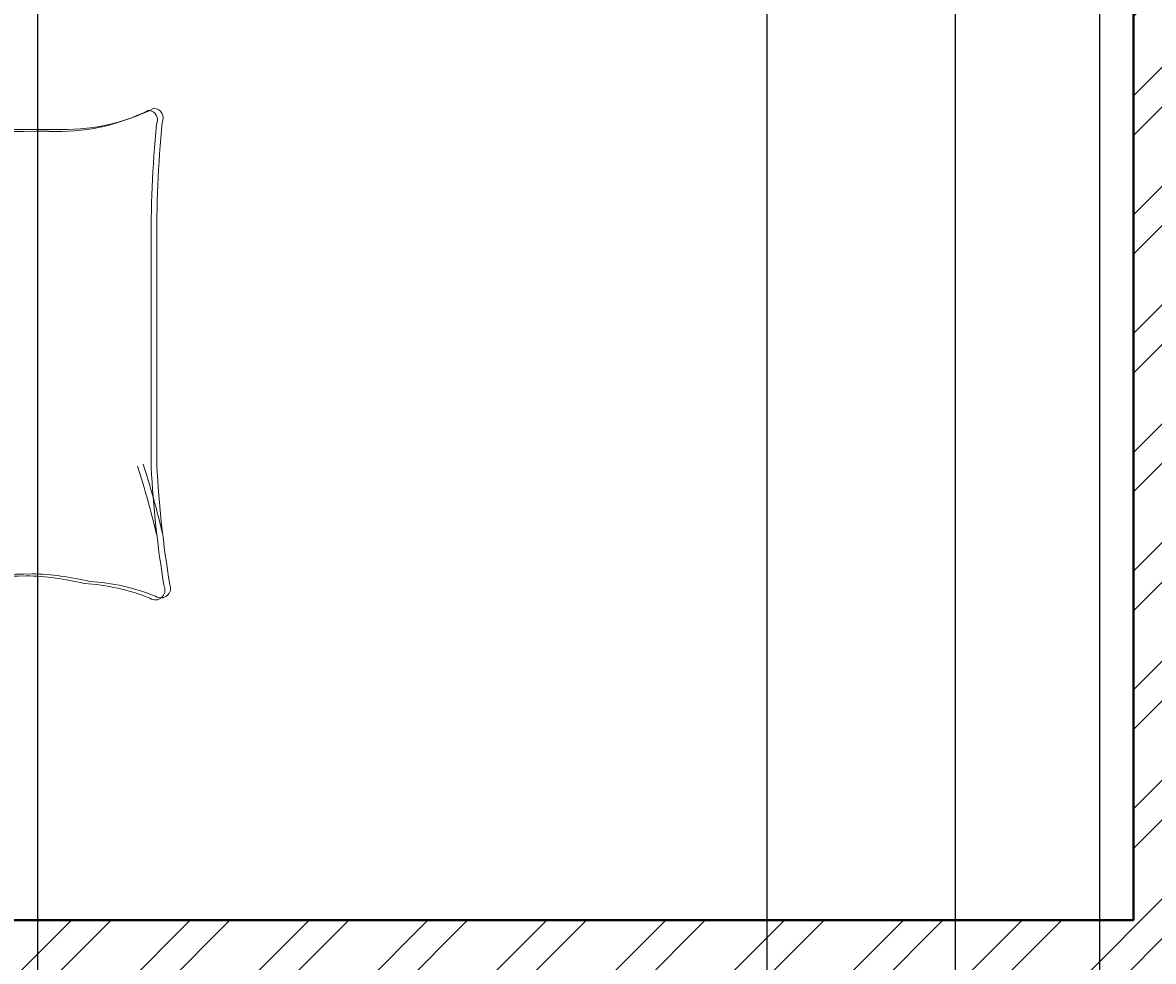
# Model space of a CAD drawing. Units: inches. Extents: x 1601 to 2297, y 1496 to 2631.
# Tile 36 of 57: x 1763 to 1891, y 2141 to 2247. Entities that reach past the tile are written whole.
import ezdxf

# ---------------------------------------------------------------- set-up
doc = ezdxf.new("R2010")
doc.units = ezdxf.units.IN
for name, color, linetype, lineweight in [('A-ANNO-DIMS', 2, 'Continuous', 18), ('A-FURN', 8, 'Continuous', 18), ('A-WALL', 7, 'Continuous', 40), ('A-WALL-PATT', 215, 'Continuous', 13)]:
    doc.layers.add(name, color=color, linetype=linetype, lineweight=lineweight)
doc.styles.get("Standard").update_dxf_attribs({"font": 'arial.ttf'})
doc.dimstyles.get("Standard").update_dxf_attribs({"dimtxt": 0.18, "dimasz": 0.18, "dimexe": 0.18, "dimexo": 0.0625, "dimgap": 0.09, "dimtad": 0, "dimtih": 1, "dimtoh": 1, "dimdec": 4, "dimzin": 0, "dimdsep": 46, "dimtxsty": 'Standard', "dimcen": 0.09, "dimadec": 0, "dimazin": 0, "dimtfac": 1, "dimtdec": 4, "dimtofl": 0, "dimtmove": 0, "dimatfit": 3, "dimfxl": 1, "dimtolj": 1, "dimtzin": 0, "dimarcsym": 0})

# ---------------------------------------------------------------- blocks, each defined once
blk = doc.blocks.new('BED-DOUBLE')
for p, q in [((27.75, 52.87), (24.5, 49.16)), ((27.75, 52.87), (24.5, 49.16)), ((27.75, 52.87), (24.5, 49.16)), ((27.75, 52.87), (24.5, 49.16)), ((28.39, 53.1), (25.13, 49.39)), ((28.39, 53.1), (25.13, 49.39)), ((28.39, 53.1), (25.13, 49.39)), ((28.39, 53.1), (25.13, 49.39)), ((29.49, 52.95), (27.75, 52.87, 3.87)), ((29.49, 52.95), (27.75, 52.87, 3.87)), ((29.49, 52.95), (27.75, 52.87, 3.87)), ((29.49, 52.95), (27.75, 52.87, 3.87)), ((28.36, 51.33), (27.75, 52.87)), ((28.36, 51.33), (27.75, 52.87)), ((28.36, 51.33), (27.75, 52.87)), ((28.36, 51.33), (27.75, 52.87)), ((30.13, 53.18), (28.39, 53.1, 3.87)), ((30.13, 53.18), (28.39, 53.1, 3.87)), ((30.13, 53.17), (28.39, 53.1, 3.87)), ((30.13, 53.17), (28.39, 53.1, 3.87)), ((29, 51.56), (28.39, 53.1)), ((29, 51.56), (28.39, 53.1)), ((29, 51.56), (28.39, 53.1)), ((29, 51.56), (28.39, 53.1)), ((0, 51.49), (0.64, 51.49)), ((0, 3.47), (0, 51.49)), ((0, 51.49), (0.64, 51.49)), ((0, 3.47), (0, 51.49)), ((0.64, 51.49), (27.25, 51.49)), ((0.64, 51.49), (27.25, 51.49)), ((0.64, 51.49), (27.25, 51.49)), ((0.64, 51.49), (27.25, 51.49)), ((2.17, 3.7), (2.17, 51.49)), ((2.17, 3.7), (2.17, 51.49)), ((2.17, 3.7), (2.17, 51.49)), ((2.17, 3.7), (2.17, 51.49)), ((28.06, 48.23), (28.36, 51.33)), ((28.06, 48.23), (28.36, 51.33)), ((28.06, 48.23), (28.36, 51.33)), ((28.06, 48.23), (28.36, 51.33)), ((28.69, 48.46), (29, 51.56)), ((28.69, 48.46), (29, 51.56)), ((28.69, 48.46), (29, 51.56)), ((28.69, 48.46), (29, 51.56)), ((0, 51.27), (26.61, 51.27)), ((0, 51.27), (26.61, 51.27)), ((0, 51.26), (26.61, 51.26)), ((0, 51.26), (26.61, 51.26)), ((1.53, 3.47), (1.53, 51.27)), ((1.53, 3.47), (1.53, 51.27)), ((1.53, 3.47), (1.53, 51.26)), ((1.53, 3.47), (1.53, 51.26)), ((2.56, 50.11), (2.46, 44.71)), ((2.56, 50.11), (2.46, 44.71)), ((2.56, 50.11), (2.46, 44.71)), ((2.56, 50.11), (2.46, 44.71)), ((2.56, 50.11), (5.77, 49.73)), ((2.56, 50.11), (5.77, 49.73)), ((2.56, 50.11), (5.77, 49.73)), ((2.56, 50.11), (5.77, 49.73)), ((3.2, 50.34), (3.1, 44.94)), ((3.2, 50.34), (3.1, 44.94)), ((3.2, 50.34), (3.1, 44.94)), ((3.2, 50.34), (3.1, 44.94)), ((3.2, 50.34), (6.41, 49.96)), ((3.2, 50.34), (6.41, 49.96)), ((3.2, 50.34), (6.41, 49.96)), ((3.2, 50.34), (6.41, 49.96)), ((5.77, 49.73), (8.34, 50.33)), ((5.77, 49.73), (8.34, 50.33)), ((5.77, 49.73), (8.34, 50.33)), ((5.77, 49.73), (8.34, 50.33)), ((6.41, 49.96), (8.98, 50.56)), ((6.41, 49.96), (8.98, 50.56)), ((6.41, 49.96), (8.98, 50.56)), ((6.41, 49.96), (8.98, 50.56)), ((11.83, 50.11), (8.26, 49.31)), ((11.83, 50.11), (8.26, 49.31)), ((11.83, 50.11), (8.26, 49.31)), ((11.83, 50.11), (8.26, 49.31)), ((8.34, 50.33), (9.38, 49.81)), ((8.34, 50.33), (9.38, 49.81)), ((8.34, 50.33), (9.38, 49.81)), ((8.34, 50.33), (9.38, 49.81)), ((12.47, 50.34), (8.9, 49.54)), ((12.47, 50.34), (8.9, 49.54)), ((12.47, 50.34), (8.9, 49.54)), ((12.47, 50.34), (8.9, 49.54)), ((8.98, 50.56), (10.02, 50.04)), ((8.98, 50.56), (10.02, 50.04)), ((8.98, 50.56), (10.02, 50.04)), ((8.98, 50.56), (10.02, 50.04)), ((13.43, 49.92), (11.83, 50.11)), ((13.43, 49.92), (11.83, 50.11)), ((13.43, 49.92), (11.83, 50.11)), ((13.43, 49.92), (11.83, 50.11)), ((14.07, 50.15), (12.47, 50.34)), ((14.07, 50.15), (12.47, 50.34)), ((14.07, 50.15), (12.47, 50.34)), ((14.07, 50.15), (12.47, 50.34)), ((16.57, 50.7), (13.43, 49.92)), ((16.57, 50.7), (13.43, 49.92)), ((16.57, 50.7), (13.43, 49.92)), ((16.57, 50.7), (13.43, 49.92)), ((17.21, 50.93), (14.07, 50.15)), ((17.21, 50.93), (14.07, 50.15)), ((17.21, 50.93), (14.07, 50.15)), ((17.21, 50.93), (14.07, 50.15)), ((16.17, 45.57), (16.57, 50.7)), ((16.17, 45.57), (16.57, 50.7)), ((16.17, 45.57), (16.57, 50.7)), ((16.17, 45.57), (16.57, 50.7)), ((16.81, 45.79), (17.21, 50.93)), ((16.81, 45.79), (17.21, 50.93)), ((16.81, 45.79), (17.21, 50.93)), ((16.81, 45.79), (17.21, 50.93)), ((8.26, 49.31), (5.58, 48.13)), ((8.26, 49.31), (5.58, 48.13)), ((8.26, 49.31), (5.58, 48.13)), ((8.26, 49.31), (5.58, 48.13)), ((8.9, 49.54), (6.22, 48.36)), ((8.9, 49.54), (6.22, 48.36)), ((8.9, 49.54), (6.22, 48.36)), ((8.9, 49.54), (6.22, 48.36)), ((24.5, 49.16), (22.33, 46.22)), ((24.5, 49.16), (22.33, 46.22)), ((24.5, 49.16), (22.33, 46.22)), ((24.5, 49.16), (22.33, 46.22)), ((25.13, 49.39), (22.97, 46.45)), ((25.13, 49.39), (22.97, 46.45)), ((25.13, 49.39), (22.97, 46.45)), ((25.13, 49.39), (22.97, 46.45)), ((28.36, 44.36), (28.06, 48.23)), ((28.36, 44.36), (28.06, 48.23)), ((28.36, 44.36), (28.06, 48.23)), ((28.36, 44.36), (28.06, 48.23)), ((29, 44.59), (28.69, 48.46)), ((29, 44.59), (28.69, 48.46)), ((29, 44.59), (28.69, 48.46)), ((29, 44.59), (28.69, 48.46)), ((22.33, 46.22), (20.32, 40.64)), ((22.33, 46.22), (20.32, 40.64)), ((22.33, 46.22), (20.32, 40.64)), ((22.33, 46.22), (20.32, 40.64)), ((22.97, 46.45), (20.96, 40.87)), ((22.97, 46.45), (20.96, 40.87)), ((22.97, 46.45), (20.96, 40.87)), ((22.97, 46.45), (20.96, 40.87)), ((2.46, 44.71), (2.54, 45.71)), ((2.46, 44.71), (2.54, 45.71)), ((2.46, 44.71), (2.54, 45.71)), ((2.46, 44.71), (2.54, 45.71)), ((2.54, 45.71), (3.07, 41.91)), ((2.54, 45.71), (3.07, 41.91)), ((2.54, 45.71), (3.07, 41.91)), ((2.54, 45.71), (3.07, 41.91)), ((3.1, 44.94), (3.18, 45.94)), ((3.1, 44.94), (3.18, 45.94)), ((3.1, 44.94), (3.18, 45.94)), ((3.1, 44.94), (3.18, 45.94)), ((3.18, 45.94), (3.71, 42.14)), ((3.18, 45.94), (3.71, 42.14)), ((3.18, 45.94), (3.71, 42.14)), ((3.18, 45.94), (3.71, 42.14)), ((16.73, 43.61), (16.17, 45.57)), ((16.73, 43.61), (16.17, 45.57)), ((16.73, 43.61), (16.17, 45.57)), ((16.73, 43.61), (16.17, 45.57)), ((17.37, 43.83), (16.81, 45.79)), ((17.37, 43.83), (16.81, 45.79)), ((17.37, 43.83), (16.81, 45.79)), ((17.37, 43.83), (16.81, 45.79)), ((16.3, 36.6), (16.73, 43.61)), ((16.3, 36.6), (16.73, 43.61)), ((16.3, 36.6), (16.73, 43.61)), ((16.3, 36.6), (16.73, 43.61)), ((16.93, 36.82), (17.37, 43.83)), ((16.93, 36.82), (17.37, 43.83)), ((16.93, 36.82), (17.37, 43.83)), ((16.93, 36.82), (17.37, 43.83)), ((28.83, 40.95), (28.36, 44.36)), ((28.83, 40.95), (28.36, 44.36)), ((28.83, 40.95), (28.36, 44.36)), ((28.83, 40.95), (28.36, 44.36)), ((29.47, 41.18), (29, 44.59)), ((29.47, 41.18), (29, 44.59)), ((29.47, 41.18), (29, 44.59)), ((29.47, 41.18), (29, 44.59)), ((3.07, 41.91), (4.42, 36.49)), ((3.07, 41.91), (4.42, 36.49)), ((3.07, 41.91), (4.42, 36.49)), ((3.07, 41.91), (4.42, 36.49)), ((3.71, 42.14), (5.06, 36.72)), ((3.71, 42.14), (5.06, 36.72)), ((3.71, 42.14), (5.06, 36.72)), ((3.71, 42.14), (5.06, 36.72)), ((30.4, 39.17), (29.47, 41.18)), ((30.4, 39.17), (29.47, 41.18)), ((30.4, 39.17), (29.47, 41.18)), ((30.4, 39.17), (29.47, 41.18)), ((20.32, 40.64), (17.38, 32.31)), ((20.32, 40.64), (17.38, 32.31)), ((20.32, 40.64), (17.38, 32.31)), ((20.32, 40.64), (17.38, 32.31)), ((20.96, 40.87), (18.02, 32.53)), ((20.96, 40.87), (18.02, 32.53)), ((20.96, 40.87), (18.02, 32.53)), ((20.96, 40.87), (18.02, 32.53)), ((29.76, 38.94), (28.83, 40.95)), ((29.76, 38.94), (28.83, 40.95)), ((29.76, 38.94), (28.83, 40.95)), ((29.76, 38.94), (28.83, 40.95)), ((79.88, 15.29), (79.88, 39.91)), ((79.88, 15.29), (79.88, 39.91)), ((79.88, 15.29), (79.88, 39.91)), ((79.88, 15.29), (79.88, 39.91)), ((3.67, 39.2), (3.08, 37.14)), ((3.67, 39.2), (3.08, 37.13)), ((3.67, 39.2), (3.08, 37.14)), ((3.67, 39.2), (3.08, 37.13)), ((4.31, 39.43), (3.72, 37.36)), ((4.31, 39.43), (3.72, 37.36)), ((4.31, 39.43), (3.72, 37.36)), ((4.31, 39.43), (3.72, 37.36)), ((30.38, 36.46), (29.76, 38.94)), ((30.38, 36.46), (29.76, 38.94)), ((30.38, 36.46), (29.76, 38.94)), ((30.38, 36.46), (29.76, 38.94)), ((31.02, 36.69), (30.4, 39.17)), ((31.02, 36.69), (30.4, 39.17)), ((31.02, 36.69), (30.4, 39.17)), ((31.02, 36.69), (30.4, 39.17)), ((79.24, 15.06), (79.24, 39.68)), ((79.24, 15.06), (79.24, 39.68)), ((79.24, 15.06), (79.24, 39.68)), ((79.24, 15.06), (79.24, 39.68)), ((3.72, 37.36), (3.18, 34.43)), ((3.72, 37.36), (3.18, 34.43)), ((3.72, 37.36), (3.18, 34.43)), ((3.72, 37.36), (3.18, 34.43)), ((3.08, 37.14), (2.54, 34.2)), ((3.08, 37.14), (2.54, 34.2)), ((3.08, 37.13), (2.54, 34.2)), ((3.08, 37.13), (2.54, 34.2)), ((15.63, 32.56), (16.3, 36.6)), ((15.63, 32.56), (16.3, 36.6)), ((15.63, 32.56), (16.3, 36.6)), ((15.63, 32.56), (16.3, 36.6)), ((16.27, 32.79), (16.93, 36.82)), ((16.27, 32.79), (16.93, 36.82)), ((16.27, 32.79), (16.93, 36.82)), ((16.27, 32.79), (16.93, 36.82)), ((23.88, 34.45), (28.36, 36.15)), ((23.88, 34.45), (28.36, 36.15)), ((23.88, 34.45), (28.36, 36.15)), ((23.88, 34.45), (28.36, 36.15)), ((24.52, 34.68), (29, 36.38)), ((24.52, 34.68), (29, 36.38)), ((24.52, 34.68), (29, 36.38)), ((24.52, 34.68), (29, 36.38)), ((28.36, 36.15), (30.38, 36.46)), ((28.36, 36.15), (30.38, 36.46)), ((28.36, 36.15), (30.38, 36.46)), ((28.36, 36.15), (30.38, 36.46)), ((29, 36.38), (31.02, 36.69)), ((29, 36.38), (31.02, 36.69)), ((29, 36.38), (31.02, 36.69)), ((29, 36.38), (31.02, 36.69)), ((18.02, 30.49), (24.52, 34.68)), ((18.02, 30.49), (24.52, 34.68)), ((18.02, 30.49), (24.52, 34.68)), ((18.02, 30.49), (24.52, 34.68)), ((2.54, 34.2), (2.56, 33.88)), ((2.54, 34.2), (2.56, 33.88)), ((2.54, 34.2), (2.56, 33.88)), ((2.54, 34.2), (2.56, 33.88)), ((2.56, 33.88), (2.98, 29.46)), ((2.56, 33.88), (2.98, 29.46)), ((2.56, 33.88), (2.98, 29.46)), ((2.56, 33.88), (2.98, 29.46)), ((3.18, 34.43), (3.2, 34.11)), ((3.18, 34.43), (3.2, 34.11)), ((3.18, 34.43), (3.2, 34.11)), ((3.18, 34.43), (3.2, 34.11)), ((3.2, 34.11), (3.62, 29.68)), ((3.2, 34.11), (3.62, 29.68)), ((3.2, 34.11), (3.62, 29.68)), ((3.2, 34.11), (3.62, 29.68)), ((16.74, 30.75), (15.45, 33.82)), ((16.74, 30.75), (15.45, 33.82)), ((16.74, 30.75), (15.45, 33.82)), ((16.74, 30.75), (15.45, 33.82)), ((17.38, 30.98), (16.09, 34.05)), ((17.38, 30.98), (16.09, 34.05)), ((17.38, 30.98), (16.09, 34.05)), ((17.38, 30.98), (16.09, 34.05)), ((17.38, 30.26), (23.88, 34.45)), ((17.38, 30.26), (23.88, 34.45)), ((17.38, 30.26), (23.88, 34.45)), ((17.38, 30.26), (23.88, 34.45)), ((17.53, 28.53), (17.38, 30.98)), ((17.53, 28.53), (17.38, 30.98)), ((17.53, 28.53), (17.38, 30.98)), ((17.53, 28.53), (17.38, 30.98)), ((3.62, 29.68), (3.13, 28.21)), ((3.62, 29.68), (3.13, 28.2)), ((3.62, 29.68), (3.13, 28.21)), ((3.62, 29.68), (3.13, 28.2)), ((16.89, 28.3), (16.74, 30.75)), ((16.89, 28.3), (16.74, 30.75)), ((16.89, 28.3), (16.74, 30.75)), ((16.89, 28.3), (16.74, 30.75)), ((2.98, 29.46), (2.49, 27.98)), ((2.98, 29.46), (2.49, 27.98)), ((2.98, 29.46), (2.49, 27.98)), ((2.98, 29.46), (2.49, 27.98)), ((3.13, 28.21), (8.51, 27.96)), ((3.13, 28.21), (8.51, 27.96)), ((3.13, 28.2), (8.51, 27.96)), ((3.13, 28.2), (8.51, 27.96)), ((13.02, 27.66), (14.86, 28.36)), ((13.02, 27.66), (14.86, 28.36)), ((13.02, 27.66), (14.86, 28.36)), ((13.02, 27.66), (14.86, 28.36)), ((14.22, 28.13), (16.89, 28.3)), ((14.22, 28.13), (16.89, 28.3)), ((14.22, 28.13), (16.89, 28.3)), ((14.22, 28.13), (16.89, 28.3)), ((14.86, 28.36), (17.53, 28.53)), ((14.86, 28.36), (17.53, 28.53)), ((14.86, 28.36), (17.53, 28.53)), ((14.86, 28.36), (17.53, 28.53)), ((2.49, 27.98), (7.87, 27.73)), ((2.49, 27.98), (7.87, 27.73)), ((2.49, 27.98), (7.87, 27.73)), ((2.49, 27.98), (7.87, 27.73)), ((7.22, 26.56), (10.4, 27.14)), ((7.22, 26.56), (10.4, 27.14)), ((7.22, 26.56), (10.4, 27.14)), ((7.22, 26.56), (10.4, 27.14)), ((7.86, 26.79), (11.04, 27.37)), ((7.86, 26.79), (11.04, 27.37)), ((7.86, 26.79), (11.04, 27.37)), ((7.86, 26.79), (11.04, 27.37)), ((7.87, 27.73), (11.08, 27.35)), ((7.87, 27.73), (11.08, 27.35)), ((7.87, 27.73), (11.08, 27.35)), ((7.87, 27.73), (11.08, 27.35)), ((8.51, 27.96), (11.72, 27.58)), ((8.51, 27.96), (11.72, 27.58)), ((8.51, 27.96), (11.72, 27.58)), ((8.51, 27.96), (11.72, 27.58)), ((10.4, 27.14), (11.7, 27.14)), ((10.4, 27.14), (11.7, 27.14)), ((10.4, 27.14), (11.7, 27.14)), ((10.4, 27.14), (11.7, 27.14)), ((11.04, 27.37), (12.34, 27.37)), ((11.04, 27.37), (12.34, 27.37)), ((11.04, 27.37), (12.34, 27.37)), ((11.04, 27.37), (12.34, 27.37)), ((11.08, 27.35), (12.38, 27.44)), ((11.08, 27.35), (12.38, 27.44)), ((11.08, 27.35), (12.38, 27.44)), ((11.08, 27.35), (12.38, 27.44)), ((11.7, 27.14), (13.58, 26.56)), ((11.7, 27.14), (13.58, 26.56)), ((11.7, 27.14), (13.58, 26.56)), ((11.7, 27.14), (13.58, 26.56)), ((11.72, 27.58), (13.02, 27.66)), ((11.72, 27.58), (13.02, 27.66)), ((11.72, 27.58), (13.02, 27.66)), ((11.72, 27.58), (13.02, 27.66)), ((12.34, 27.37), (14.22, 26.79)), ((12.34, 27.37), (14.22, 26.79)), ((12.34, 27.37), (14.22, 26.79)), ((12.34, 27.37), (14.22, 26.79)), ((12.38, 27.44), (14.22, 28.13)), ((12.38, 27.44), (14.22, 28.13)), ((12.38, 27.44), (14.22, 28.13)), ((12.38, 27.44), (14.22, 28.13)), ((1.87, 25.98), (7.22, 26.56)), ((1.87, 25.98), (7.22, 26.56)), ((1.87, 25.98), (7.22, 26.56)), ((1.87, 25.98), (7.22, 26.56)), ((2.45, 24.54), (1.87, 25.98)), ((2.45, 24.54), (1.87, 25.98)), ((2.45, 24.54), (1.87, 25.98)), ((2.45, 24.54), (1.87, 25.98)), ((2.51, 26.21), (7.86, 26.79)), ((2.51, 26.21), (7.86, 26.79)), ((2.51, 26.21), (7.86, 26.79)), ((2.51, 26.21), (7.86, 26.79)), ((3.09, 24.77), (2.51, 26.21)), ((3.09, 24.76), (2.51, 26.21)), ((3.09, 24.77), (2.51, 26.21)), ((3.09, 24.76), (2.51, 26.21)), ((13.58, 26.56), (16.26, 26.56)), ((13.58, 26.56), (16.26, 26.56)), ((13.58, 26.56), (16.26, 26.56)), ((13.58, 26.56), (16.26, 26.56)), ((14.22, 26.79), (16.9, 26.79)), ((14.22, 26.79), (16.9, 26.79)), ((14.22, 26.79), (16.9, 26.79)), ((14.22, 26.79), (16.9, 26.79)), ((16.26, 26.56), (16.26, 24.1)), ((16.26, 26.56), (16.26, 24.1)), ((16.26, 26.56), (16.26, 24.1)), ((16.26, 26.56), (16.26, 24.1)), ((16.9, 26.79), (16.9, 24.33)), ((16.9, 26.79), (16.9, 24.33)), ((16.9, 26.79), (16.9, 24.33)), ((16.9, 26.79), (16.9, 24.33)), ((2.3, 20.09), (2.45, 24.54)), ((2.3, 20.09), (2.45, 24.54)), ((2.3, 20.09), (2.45, 24.54)), ((2.3, 20.09), (2.45, 24.54)), ((2.94, 20.32), (3.09, 24.77)), ((2.94, 20.32), (3.09, 24.77)), ((2.94, 20.32), (3.09, 24.76)), ((2.94, 20.32), (3.09, 24.76)), ((16.17, 19.38), (16.57, 24.52)), ((16.17, 19.38), (16.57, 24.52)), ((16.17, 19.38), (16.57, 24.52)), ((16.17, 19.38), (16.57, 24.52)), ((16.81, 19.61), (17.21, 24.74)), ((16.81, 19.61), (17.21, 24.74)), ((16.81, 19.61), (17.21, 24.74)), ((16.81, 19.61), (17.21, 24.74)), ((16.26, 24.1), (15.17, 20.96)), ((16.26, 24.1), (15.17, 20.96)), ((16.26, 24.1), (15.17, 20.96)), ((16.26, 24.1), (15.17, 20.96)), ((16.9, 24.33), (15.81, 21.19)), ((16.9, 24.33), (15.81, 21.19)), ((16.9, 24.33), (15.81, 21.19)), ((16.9, 24.33), (15.81, 21.19)), ((2.3, 19.77), (2.3, 20.09)), ((2.3, 19.77), (2.3, 20.09)), ((2.3, 19.77), (2.3, 20.09)), ((2.3, 19.77), (2.3, 20.09)), ((3.03, 16.88), (2.3, 19.77)), ((3.03, 16.88), (2.3, 19.77)), ((3.03, 16.88), (2.3, 19.77)), ((3.03, 16.88), (2.3, 19.77)), ((2.94, 20), (2.94, 20.32)), ((2.94, 20), (2.94, 20.32)), ((2.94, 20), (2.94, 20.32)), ((2.94, 20), (2.94, 20.32)), ((3.67, 17.11), (2.94, 20)), ((3.67, 17.11), (2.94, 20)), ((3.67, 17.11), (2.94, 20)), ((3.67, 17.11), (2.94, 20)), ((16.73, 17.42), (16.17, 19.38)), ((16.73, 17.42), (16.17, 19.38)), ((16.73, 17.42), (16.17, 19.38)), ((16.73, 17.42), (16.17, 19.38)), ((17.37, 17.65), (16.81, 19.61)), ((17.37, 17.65), (16.81, 19.61)), ((17.37, 17.65), (16.81, 19.61)), ((17.37, 17.65), (16.81, 19.61)), ((3.75, 14.85), (3.03, 16.88)), ((3.75, 14.85), (3.03, 16.88)), ((3.75, 14.85), (3.03, 16.88)), ((3.75, 14.85), (3.03, 16.88)), ((3.32, 12.11), (4.33, 17.6)), ((3.32, 12.11), (4.33, 17.6)), ((3.32, 12.11), (4.33, 17.6)), ((3.32, 12.11), (4.33, 17.6)), ((4.39, 15.08), (3.67, 17.11)), ((4.39, 15.08), (3.67, 17.11)), ((4.39, 15.08), (3.67, 17.11)), ((4.39, 15.08), (3.67, 17.11)), ((3.96, 12.34), (4.97, 17.83)), ((3.96, 12.34), (4.97, 17.83)), ((3.96, 12.34), (4.97, 17.83)), ((3.96, 12.34), (4.97, 17.83)), ((16.3, 10.41), (16.73, 17.42)), ((16.3, 10.41), (16.73, 17.42)), ((16.3, 10.41), (16.73, 17.42)), ((16.3, 10.41), (16.73, 17.42)), ((16.93, 10.64), (17.37, 17.65)), ((16.93, 10.64), (17.37, 17.65)), ((16.93, 10.64), (17.37, 17.65)), ((16.93, 10.64), (17.37, 17.65)), ((3.03, 8.28), (3.32, 12.11)), ((3.03, 8.28), (3.32, 12.11)), ((3.03, 8.28), (3.32, 12.11)), ((3.03, 8.28), (3.32, 12.11)), ((3.67, 8.51), (3.96, 12.34)), ((3.67, 8.51), (3.96, 12.34)), ((3.67, 8.51), (3.96, 12.34)), ((3.67, 8.51), (3.96, 12.34)), ((15.63, 6.38), (16.3, 10.41)), ((15.63, 6.38), (16.3, 10.41)), ((15.63, 6.38), (16.3, 10.41)), ((15.63, 6.38), (16.3, 10.41)), ((16.27, 6.61), (16.93, 10.64)), ((16.27, 6.61), (16.93, 10.64)), ((16.27, 6.61), (16.93, 10.64)), ((16.27, 6.61), (16.93, 10.64)), ((16.3, 10.41), (16.62, 9.28)), ((16.3, 10.41), (16.62, 9.28)), ((16.3, 10.41), (16.62, 9.28)), ((16.3, 10.41), (16.62, 9.28)), ((16.93, 10.64), (17.26, 9.51)), ((16.93, 10.64), (17.26, 9.51)), ((16.93, 10.64), (17.26, 9.51)), ((16.93, 10.64), (17.26, 9.51)), ((16.62, 9.28), (17.34, 4.18)), ((16.62, 9.28), (17.34, 4.18)), ((16.62, 9.28), (17.34, 4.18)), ((16.62, 9.28), (17.34, 4.18)), ((17.26, 9.51), (17.98, 4.41)), ((17.26, 9.51), (17.98, 4.41)), ((17.26, 9.51), (17.98, 4.41)), ((17.26, 9.51), (17.98, 4.41)), ((3.01, 8.18), (3.03, 8.28)), ((3.01, 8.18), (3.03, 8.28)), ((3.01, 8.18), (3.03, 8.28)), ((3.01, 8.18), (3.03, 8.28)), ((3.34, 3.9), (3.01, 8.18)), ((3.34, 3.9), (3.01, 8.18)), ((3.34, 3.9), (3.01, 8.18)), ((3.34, 3.9), (3.01, 8.18)), ((3.65, 8.41), (3.67, 8.51)), ((3.65, 8.41), (3.67, 8.51)), ((3.65, 8.41), (3.67, 8.51)), ((3.65, 8.41), (3.67, 8.51)), ((3.98, 4.13), (3.65, 8.41)), ((3.98, 4.13), (3.65, 8.41)), ((3.98, 4.13), (3.65, 8.41)), ((3.98, 4.13), (3.65, 8.41)), ((8.95, 5.05), (6.21, 6.06)), ((8.95, 5.05), (6.21, 6.06)), ((8.95, 5.05), (6.21, 6.06)), ((8.95, 5.05), (6.21, 6.06)), ((9.59, 5.28), (6.85, 6.29)), ((9.59, 5.28), (6.85, 6.29)), ((9.59, 5.28), (6.85, 6.29)), ((9.59, 5.28), (6.85, 6.29)), ((13.21, 4.7), (9.59, 5.28)), ((13.21, 4.7), (9.59, 5.28)), ((13.21, 4.7), (9.59, 5.28)), ((13.21, 4.7), (9.59, 5.28)), ((3.32, 3.89), (6.5, 4.47)), ((3.32, 3.89), (6.5, 4.47)), ((3.32, 3.89), (6.5, 4.47)), ((3.32, 3.89), (6.5, 4.47)), ((3.96, 4.12), (7.14, 4.7)), ((3.96, 4.12), (7.14, 4.7)), ((3.96, 4.12), (7.14, 4.7)), ((3.96, 4.12), (7.14, 4.7)), ((6.5, 4.47), (9.1, 4.04)), ((6.5, 4.47), (9.1, 4.04)), ((6.5, 4.47), (9.1, 4.04)), ((6.5, 4.47), (9.1, 4.04)), ((7.14, 4.7), (9.74, 4.27)), ((7.14, 4.7), (9.74, 4.27)), ((7.14, 4.7), (9.74, 4.27)), ((7.14, 4.7), (9.74, 4.27)), ((12.57, 4.47), (8.95, 5.05)), ((12.57, 4.47), (8.95, 5.05)), ((12.57, 4.47), (8.95, 5.05)), ((12.57, 4.47), (8.95, 5.05)), ((9.1, 4.04), (10.11, 4.62)), ((9.1, 4.04), (10.11, 4.62)), ((9.1, 4.04), (10.11, 4.62)), ((9.1, 4.04), (10.11, 4.62)), ((9.74, 4.27), (10.75, 4.85)), ((9.74, 4.27), (10.75, 4.85)), ((9.74, 4.27), (10.75, 4.85)), ((9.74, 4.27), (10.75, 4.85)), ((14.16, 4.76), (12.57, 4.47)), ((14.16, 4.76), (12.57, 4.47)), ((14.16, 4.76), (12.57, 4.47)), ((14.16, 4.76), (12.57, 4.47)), ((14.8, 4.99), (13.21, 4.7)), ((14.8, 4.99), (13.21, 4.7)), ((14.8, 4.99), (13.21, 4.7)), ((14.8, 4.99), (13.21, 4.7)), ((17.34, 4.18), (14.16, 4.76)), ((17.34, 4.18), (14.16, 4.76)), ((17.34, 4.18), (14.16, 4.76)), ((17.34, 4.18), (14.16, 4.76)), ((17.98, 4.41), (14.8, 4.99)), ((17.98, 4.41), (14.8, 4.99)), ((17.98, 4.41), (14.8, 4.99)), ((17.98, 4.41), (14.8, 4.99)), ((18.11, 3.47), (0, 3.47)), ((18.11, 3.47), (0, 3.47)), ((18.11, 3.47), (0, 3.47)), ((18.11, 3.47), (0, 3.47)), ((18.75, 3.7), (0.64, 3.7)), ((18.75, 3.7), (0.64, 3.7)), ((18.75, 3.7), (0.64, 3.7)), ((18.75, 3.7), (0.64, 3.7))]:
    blk.add_line(p, q)
for centre, radius, start, end in [((68.67, 76.16), 23.07, 267.4714, 296.4681), ((68.67, 76.16), 23.07, 267.4714, 296.4681), ((68.67, 76.16), 23.07, 267.4714, 296.4681), ((68.67, 76.16), 23.07, 267.4714, 296.4681), ((69.31, 76.39), 23.07, 267.4714, 296.4681), ((69.31, 76.39), 23.07, 267.4714, 296.4681), ((69.31, 76.39), 23.07, 267.4714, 296.4681), ((69.31, 76.39), 23.07, 267.4714, 296.4681), ((78.87, 54.41), 1.1, 332.6588, 86.02), ((78.87, 54.41), 1.1, 332.6588, 86.02), ((78.87, 54.41), 1.1, 332.6588, 86.02), ((78.87, 54.41), 1.1, 332.6588, 86.02), ((79.51, 54.64), 1.1, 332.6588, 86.02), ((79.51, 54.64), 1.1, 332.6588, 86.02), ((79.51, 54.64), 1.1, 332.6588, 86.02), ((79.51, 54.64), 1.1, 332.6588, 86.02), ((212.28, 41.15), 133.04, 174.4998, 180.6351), ((212.28, 41.15), 133.04, 174.4998, 180.6351), ((212.28, 41.15), 133.04, 174.4998, 180.6351), ((212.28, 41.15), 133.04, 174.4998, 180.6351), ((212.92, 41.38), 133.04, 174.4998, 180.6351), ((212.92, 41.38), 133.04, 174.4998, 180.6351), ((212.92, 41.38), 133.04, 174.4998, 180.6351), ((212.92, 41.38), 133.04, 174.4998, 180.6351), ((-6.66, 51.33), 36.18, 349.8763, 2.5657), ((-6.66, 51.33), 36.18, 349.8763, 2.5657), ((-6.66, 51.33), 36.18, 349.8763, 2.5657), ((-6.66, 51.33), 36.18, 349.8763, 2.5657), ((36.31, 182.27), 129.5, 266.9791, 273.8365), ((36.31, 182.27), 129.5, 266.9791, 273.8365), ((36.31, 182.27), 129.5, 266.9791, 273.8365), ((36.31, 182.27), 129.5, 266.9791, 273.8365), ((-6.02, 51.56), 36.18, 349.8763, 2.5657), ((-6.02, 51.56), 36.18, 349.8763, 2.5657), ((-6.02, 51.56), 36.18, 349.8763, 2.5657), ((-6.02, 51.56), 36.18, 349.8763, 2.5657), ((36.95, 182.49), 129.5, 266.9791, 273.8365), ((36.95, 182.49), 129.5, 266.9791, 273.8365), ((36.95, 182.49), 129.5, 266.9791, 273.8365), ((36.95, 182.49), 129.5, 266.9791, 273.8365), ((67.82, -4508.74), 4561.86, 90.00217, 90.28689), ((67.82, -4508.74), 4561.86, 90.00217, 90.28689), ((67.82, -4508.74), 4561.86, 90.00217, 90.28689), ((67.82, -4508.74), 4561.86, 90.00217, 90.28689), ((68.46, -4508.52), 4561.86, 90.00217, 90.28689), ((68.46, -4508.52), 4561.86, 90.00217, 90.28689), ((68.46, -4508.52), 4561.86, 90.00217, 90.28689), ((68.46, -4508.52), 4561.86, 90.00217, 90.28689), ((35.07, 43.74), 6.22, 168.6608, 203.7384), ((35.07, 43.74), 6.22, 168.6608, 203.7384), ((35.07, 43.74), 6.22, 168.6608, 203.7384), ((35.07, 43.74), 6.22, 168.6608, 203.7384), ((35.71, 43.97), 6.22, 168.6608, 203.7384), ((35.71, 43.97), 6.22, 168.6608, 203.7384), ((35.71, 43.97), 6.22, 168.6608, 203.7384), ((35.71, 43.97), 6.22, 168.6608, 203.7384), ((1.48, 31.15), 29.65, 10.6617, 19.8806), ((1.48, 31.15), 29.65, 10.6617, 19.8806), ((1.48, 31.15), 29.65, 10.6617, 19.8806), ((1.48, 31.15), 29.65, 10.6617, 19.8806), ((2.12, 31.38), 29.65, 10.6617, 19.8806), ((2.12, 31.38), 29.65, 10.6617, 19.8806), ((2.12, 31.38), 29.65, 10.6617, 19.8806), ((2.12, 31.38), 29.65, 10.6617, 19.8806), ((156.32, 17.76), 129.02, 171.7845, 186.9006), ((156.32, 17.76), 129.02, 171.7845, 186.9006), ((156.32, 17.76), 129.02, 171.7845, 186.9006), ((156.32, 17.76), 129.02, 171.7845, 186.9006), ((156.96, 17.98), 129.02, 171.7845, 186.9006), ((156.96, 17.98), 129.02, 171.7845, 186.9006), ((156.96, 17.98), 129.02, 171.7845, 186.9006), ((156.96, 17.98), 129.02, 171.7845, 186.9006), ((30.44, 36.64), 0.185, 250.2464, 1.1377), ((30.44, 36.64), 0.185, 250.2464, 1.1377), ((30.44, 36.64), 0.185, 250.2464, 1.1377), ((30.44, 36.64), 0.185, 250.2464, 1.1377), ((31.08, 36.86), 0.185, 250.2464, 1.1377), ((31.08, 36.86), 0.185, 250.2464, 1.1377), ((31.08, 36.86), 0.185, 250.2464, 1.1377), ((31.08, 36.86), 0.185, 250.2464, 1.1377), ((182.05, 21.36), 164.97, 176.0865, 186.7821), ((182.05, 21.36), 164.97, 176.0865, 186.7821), ((182.05, 21.36), 164.97, 176.0865, 186.7821), ((182.05, 21.36), 164.97, 176.0865, 186.7821), ((182.69, 21.59), 164.97, 176.0865, 186.7821), ((182.69, 21.59), 164.97, 176.0865, 186.7821), ((182.69, 21.59), 164.97, 176.0865, 186.7821), ((182.69, 21.59), 164.97, 176.0865, 186.7821), ((-23.07, -16.99), 106.46, 13.3832, 17.7053), ((-23.07, -16.99), 106.46, 13.3832, 17.7053), ((-23.07, -16.99), 106.46, 13.3832, 17.7053), ((-23.07, -16.99), 106.46, 13.3832, 17.7053), ((-23.71, -17.22), 106.46, 13.3832, 17.7053), ((-23.71, -17.22), 106.46, 13.3832, 17.7053), ((-23.71, -17.22), 106.46, 13.3832, 17.7053), ((-23.71, -17.22), 106.46, 13.3832, 17.7053), ((200.84, 21.43), 121.76, 182.9958, 189.4091), ((200.84, 21.43), 121.76, 182.9958, 189.4091), ((200.84, 21.43), 121.76, 182.9958, 189.4091), ((200.84, 21.43), 121.76, 182.9958, 189.4091), ((201.48, 21.65), 121.76, 182.9958, 189.4091), ((201.48, 21.65), 121.76, 182.9958, 189.4091), ((201.48, 21.65), 121.76, 182.9958, 189.4091), ((201.48, 21.65), 121.76, 182.9958, 189.4091), ((31.17, -167.31), 170.11, 88.4762, 91.0082), ((31.17, -167.31), 170.11, 88.4762, 91.0082), ((31.17, -167.31), 170.11, 88.4762, 91.0082), ((31.17, -167.31), 170.11, 88.4762, 91.0082), ((31.81, -167.08), 170.11, 88.4762, 91.0082), ((31.81, -167.08), 170.11, 88.4762, 91.0082), ((31.81, -167.08), 170.11, 88.4762, 91.0082), ((31.81, -167.08), 170.11, 88.4762, 91.0082), ((50.61, 484.82), 482.31, 268.2277, 271.7185), ((50.61, 484.82), 482.31, 268.2277, 271.7185), ((50.61, 484.82), 482.31, 268.2277, 271.7185), ((50.61, 484.82), 482.31, 268.2277, 271.7185), ((51.25, 485.05), 482.31, 268.2277, 271.7185), ((51.25, 485.05), 482.31, 268.2277, 271.7185), ((51.25, 485.05), 482.31, 268.2277, 271.7185), ((51.25, 485.05), 482.31, 268.2277, 271.7185), ((64.51, -26.9), 29.63, 76.0648, 88.9113), ((64.51, -26.9), 29.63, 76.0648, 88.9113), ((64.51, -26.9), 29.63, 76.0648, 88.9113), ((64.51, -26.9), 29.63, 76.0648, 88.9113), ((65.15, -26.67), 29.63, 76.0648, 88.9113), ((65.15, -26.67), 29.63, 76.0648, 88.9113), ((65.15, -26.67), 29.63, 76.0648, 88.9113), ((65.15, -26.67), 29.63, 76.0648, 88.9113), ((20.1, 85.16), 83.31, 268.7218, 275.604), ((20.1, 85.16), 83.31, 268.7218, 275.604), ((20.1, 85.16), 83.31, 268.7218, 275.604), ((20.1, 85.16), 83.31, 268.7218, 275.604), ((20.74, 85.39), 83.31, 268.7218, 275.604), ((20.74, 85.39), 83.31, 268.7218, 275.604), ((20.74, 85.39), 83.31, 268.7218, 275.604), ((20.74, 85.39), 83.31, 268.7218, 275.604), ((70.28, -21.66), 23.56, 67.9751, 86.652), ((70.28, -21.66), 23.56, 67.9751, 86.652), ((70.28, -21.66), 23.56, 67.9751, 86.652), ((70.28, -21.66), 23.56, 67.9751, 86.652), ((70.91, -21.43), 23.56, 67.9751, 86.652), ((70.91, -21.43), 23.56, 67.9751, 86.652), ((70.91, -21.43), 23.56, 67.9751, 86.652), ((70.91, -21.43), 23.56, 67.9751, 86.652), ((79.72, 1.09), 1.09, 236.1736, 23.4781), ((79.72, 1.09), 1.09, 236.1736, 23.4781), ((79.72, 1.09), 1.09, 236.1736, 23.4781), ((79.72, 1.09), 1.09, 236.1736, 23.4781), ((80.36, 1.32), 1.09, 236.1736, 23.4781), ((80.36, 1.32), 1.09, 236.1736, 23.4781), ((80.36, 1.32), 1.09, 236.1736, 23.4781), ((80.36, 1.32), 1.09, 236.1736, 23.4781)]:
    blk.add_arc(centre, radius, start, end)
blk = doc.blocks.new('*D33')
at = {"layer": 'A-ANNO-DIMS', "color": 0, "lineweight": -2, "transparency": 16777216}
for p, q in [((1764.34, 2136.39), (1764.34, 2581.06)), ((1764.52, 2580.88), (1816.06, 2580.88)), ((1868.16, 2580.88), (1816.62, 2580.88)), ((1868.34, 2136.39), (1868.34, 2581.06))]:
    blk.add_line(p, q, dxfattribs=at)
at = {"layer": 'A-ANNO-DIMS', "color": 0, "transparency": 16777216}
for points in [[(1764.52, 2580.91), (1764.52, 2580.85), (1764.34, 2580.88)], [(1868.16, 2580.91), (1868.16, 2580.85), (1868.34, 2580.88)]]:
    blk.add_solid(points, dxfattribs=at)
at = {"layer": 'Defpoints', "color": 0, "transparency": 16777216}
for p in [(1868.34, 2580.88), (1764.34, 2136.33), (1868.34, 2136.33)]:
    blk.add_point(p, dxfattribs=at)
at = {"layer": 'A-ANNO-DIMS', "color": 0, "transparency": 16777216, "insert": (1816.34, 2580.88), "char_height": 0.18, "attachment_point": 5}
blk.add_mtext('\\A1;104', dxfattribs=at)
blk = doc.blocks.new('*D46')
at = {"layer": 'A-ANNO-DIMS', "color": 0, "lineweight": -2, "transparency": 16777216}
for p, q in [((1846.99, 2347.76), (1846.99, 1513.75)), ((1884.68, 2347.76), (1884.68, 1513.75)), ((1847.17, 1513.93), (1865.44, 1513.93)), ((1884.5, 1513.93), (1866.23, 1513.93))]:
    blk.add_line(p, q, dxfattribs=at)
at = {"layer": 'A-ANNO-DIMS', "color": 0, "transparency": 16777216}
for points in [[(1847.17, 1513.96), (1847.17, 1513.9), (1846.99, 1513.93)], [(1884.5, 1513.96), (1884.5, 1513.9), (1884.68, 1513.93)]]:
    blk.add_solid(points, dxfattribs=at)
at = {"layer": 'Defpoints', "color": 0, "transparency": 16777216}
for p in [(1846.99, 2347.83), (1884.68, 2347.83), (1884.68, 1513.93)]:
    blk.add_point(p, dxfattribs=at)
at = {"layer": 'A-ANNO-DIMS', "color": 0, "transparency": 16777216, "insert": (1865.84, 1513.93), "char_height": 0.18, "attachment_point": 5}
blk.add_mtext('\\A1;37.68', dxfattribs=at)

msp = doc.modelspace()

# ---------------------------------------------------------------- hatches: boundary and pattern name
at = {"layer": 'A-WALL-PATT'}
h = msp.add_hatch(dxfattribs=at)
h.set_pattern_fill('ANSI32', color=256)
h.paths.add_polyline_path([(1973.9371, 2211.3254), (1893.0373, 2211.3254), (1893.0373, 2287.8254), (1884.6167, 2287.8254), (1884.6167, 2285.5754), (1884.6167, 2283.3254), (1888.5373, 2283.3254), (1888.5373, 2145.3254), (1695.0373, 2145.3254), (1695.0373, 2173.8724), (1690.5373, 2173.8724), (1686.0373, 2173.8724), (1686.0373, 2136.3254), (1722.5687, 2136.3254), (1722.5687, 2117.4352), (1731.5687, 2117.4352), (1731.5687, 2136.3254), (1893.0373, 2136.3254), (1893.0373, 2202.3254), (1959.0373, 2202.3254), (1959.0373, 2182.1303), (1968.0373, 2182.1303), (1968.0373, 2202.3254), (1973.9371, 2202.3254)])
h.paths.add_polyline_path([(2094.0373, 2274.6364), (2096.4294, 2274.6364), (2096.4294, 2276.8864), (2096.4294, 2279.1364), (2094.0373, 2279.1364), (2094.0373, 2290.8254), (2094.0373, 2295.3254), (2089.5373, 2295.3254), (2089.5373, 2230.8254), (2035.5373, 2230.8254), (2035.5373, 2299.8254), (2031.0373, 2299.8254), (2031.0373, 2211.3254), (2023.0065, 2211.3254), (2023.0065, 2202.3254), (2031.0373, 2202.3254), (2031.0373, 2140.8254), (1968.0373, 2140.8254), (1968.0373, 2145.9106), (1963.5373, 2145.9106), (1959.0373, 2145.9106), (1959.0373, 2116.839), (1963.5373, 2116.839), (1968.0373, 2116.839), (1968.0373, 2131.8254), (2031.0373, 2131.8254), (2031.0373, 2094.3254), (2031.0373, 2085.3254), (2031.0373, 2056.8254), (1968.0373, 2056.8254), (1968.0373, 2070.4947), (1963.5373, 2070.4947), (1959.0373, 2070.4947), (1959.0373, 2040.3029), (1968.0373, 2040.3029), (1968.0373, 2047.8254), (2031.0373, 2047.8254), (2031.0373, 1983.3254), (2031.0373, 1978.8254), (2021.1979, 1978.8254), (2021.1979, 1974.3254), (2031.0373, 1974.3254), (2031.0373, 1954.3528), (2035.5373, 1954.3528), (2035.5373, 1974.3254), (2035.5373, 1981.8254), (2055.5513, 1981.8254), (2055.5513, 1986.3254), (2035.5373, 1986.3254), (2035.5373, 2047.8254), (2040.0373, 2047.8254), (2040.0373, 2085.3254), (2040.0373, 2094.3254), (2040.0373, 2140.8254), (2035.5373, 2140.8254), (2035.5373, 2226.3254), (2089.5373, 2226.3254), (2094.0373, 2226.3254)])
h.paths.add_polyline_path([(2226.0373, 2230.8254), (2134.5373, 2230.8254), (2134.5373, 2233.5437), (2130.0373, 2233.5437), (2130.0373, 2226.3254), (2134.5373, 2226.3254), (2226.0373, 2226.3254)])
h.paths.add_polyline_path([(1807.1169, 1573.5395), (2055.0405, 1573.5395), (2055.0405, 1610.6322), (1807.1169, 1610.6322)], flags=9)
h.paths.add_polyline_path([(1841.1631, 1712.7967), (1870.3957, 1712.7967), (1870.3957, 1731.454), (1841.1631, 1731.454)], flags=9)
h.paths.add_polyline_path([(2144.3862, 1772.185), (2191.0233, 1772.185), (2191.0233, 1790.8423), (2144.3862, 1790.8423)], flags=9)
h.paths.add_polyline_path([(2143.0128, 1827.3312), (2177.9958, 1827.3312), (2177.9958, 1845.9886), (2143.0128, 1845.9886)], flags=9)
h.paths.add_polyline_path([(2041.2439, 1833.5691), (2070.8516, 1833.5691), (2070.8516, 1852.2264), (2041.2439, 1852.2264)], flags=9)
h.paths.add_polyline_path([(2097.2791, 1947.0598), (2134.2061, 1947.0598), (2134.2061, 1965.7171), (2097.2791, 1965.7171)], flags=9)
h.paths.add_polyline_path([(2214.995, 1904.3124), (2214.995, 1942.2899), (2196.3376, 1942.2899), (2196.3376, 1904.3124)], flags=9)
h.paths.add_polyline_path([(2186.6284, 2043.8031), (2219.7935, 2043.8031), (2219.7935, 2062.4605), (2186.6284, 2062.4605)], flags=9)
h.paths.add_polyline_path([(2064.0877, 2031.616), (2097.4949, 2031.616), (2097.4949, 2050.2734), (2064.0877, 2050.2734)], flags=9)
h.paths.add_polyline_path([(1973.1349, 1986.0688), (2008.4009, 1986.0688), (2008.4009, 2004.7261), (1973.1349, 2004.7261)], flags=25)
h.paths.add_polyline_path([(1976.3676, 2106.9635), (2005.7469, 2106.9635), (2005.7469, 2125.6209), (1976.3676, 2125.6209)], flags=25)
h.paths.add_polyline_path([(1991.7852, 2180.4863), (2027.0513, 2180.4863), (2027.0513, 2199.1437), (1991.7852, 2199.1437)], flags=25)
h.paths.add_polyline_path([(2106.1801, 2187.9359), (2152.2101, 2187.9359), (2152.2101, 2206.5932), (2106.1801, 2206.5932)], flags=9)
h.paths.add_polyline_path([(2148.6686, 2262.2542), (2182.318, 2262.2542), (2182.318, 2280.9115), (2148.6686, 2280.9115)], flags=9)
h.paths.add_polyline_path([(2041.6327, 2252.8147), (2071.2405, 2252.8147), (2071.2405, 2271.4721), (2041.6327, 2271.4721)], flags=25)
h.paths.add_polyline_path([(2063.9734, 2375.4265), (2100.9004, 2375.4265), (2100.9004, 2394.0839), (2063.9734, 2394.0839)], flags=9)
h.paths.add_polyline_path([(2216.4955, 2330.9748), (2216.4955, 2370.2654), (2197.8381, 2370.2654), (2197.8381, 2330.9748)], flags=9)
h.paths.add_polyline_path([(2179.1416, 2485.8687), (2212.3067, 2485.8687), (2212.3067, 2504.5261), (2179.1416, 2504.5261)], flags=9)
h.paths.add_polyline_path([(2078.7442, 2471.1516), (2112.1514, 2471.1516), (2112.1514, 2489.809), (2078.7442, 2489.809)], flags=9)
h.paths.add_polyline_path([(1915.9631, 2329.4668), (1952.8902, 2329.4668), (1952.8902, 2348.1241), (1915.9631, 2348.1241)], flags=9)
h.paths.add_polyline_path([(1904.3189, 2499.6709), (1940.4512, 2499.6709), (1940.4512, 2518.3282), (1904.3189, 2518.3282)], flags=9)
h.paths.add_polyline_path([(1892.3665, 2100.4595), (1925.6374, 2100.4595), (1925.6374, 2119.1169), (1892.3665, 2119.1169)], flags=9)
h.paths.add_polyline_path([(1909.2984, 1805.9631), (1946.2254, 1805.9631), (1946.2254, 1824.6205), (1909.2984, 1824.6205)], flags=9)
h.paths.add_polyline_path([(1934.6056, 1658.616), (1970.738, 1658.616), (1970.738, 1677.2733), (1934.6056, 1677.2733)], flags=9)
h.paths.add_polyline_path([(1711.2052, 1789.8902), (1750.0456, 1789.8902), (1750.0456, 1808.5476), (1711.2052, 1808.5476)], flags=9)
h.paths.add_polyline_path([(1742.7874, 1854.6743), (1771.9449, 1854.6743), (1771.9449, 1873.3317), (1742.7874, 1873.3317)], flags=9)
h.paths.add_polyline_path([(1807.3592, 1997.7912), (1850.1116, 1997.7912), (1850.1116, 2016.4486), (1807.3592, 2016.4486)], flags=9)
h.paths.add_polyline_path([(1717.4579, 2237.7844), (1760.2103, 2237.7844), (1760.2103, 2256.4417), (1717.4579, 2256.4417)], flags=25)
h.paths.add_polyline_path([(1780.9285, 2324.0623), (1810.086, 2324.0623), (1810.086, 2342.7197), (1780.9285, 2342.7197)], flags=9)
h.paths.add_polyline_path([(1837.696, 2449.2024), (1866.9286, 2449.2024), (1866.9286, 2467.8598), (1837.696, 2467.8598)], flags=9)
h.paths.add_polyline_path([(1712.7752, 2484.9404), (1751.6156, 2484.9404), (1751.6156, 2503.5977), (1712.7752, 2503.5977)], flags=9)

# ---------------------------------------------------------------- linework, layer by layer
at = {"layer": 'A-WALL'}
for p in [(1888.5373, 2283.3254), (1695.0373, 2145.3254)]:
    msp.add_line(p, (1888.5373, 2145.3254), dxfattribs=at)

# ---------------------------------------------------------------- block references
at = {"layer": 'A-FURN'}
msp.add_blockref('BED-DOUBLE', (1697.9442, 2181.628), dxfattribs=at)

# ---------------------------------------------------------------- dimensions: what is measured, and where the dimension line sits
at = {"layer": 'A-ANNO-DIMS'}
for base, p1, p2, override, picture, middle in [((1868.3371, 2580.8754), (1764.3371, 2136.3254), (1868.3371, 2136.3254), {"dimdec": 0, "dimlfac": 1, "dimrnd": 0, "dimzin": 0, "dimdsep": 46, "dimlunit": 2}, '*D33', (1816.3371, 2580.8754)), ((1884.6773, 1513.9279), (1846.9946, 2347.8254), (1884.6773, 2347.8254), {"dimdec": 2, "dimlfac": 1, "dimrnd": 0, "dimzin": 0, "dimdsep": 46, "dimlunit": 2}, '*D46', (1865.836, 1513.9279))]:
    dim = msp.add_linear_dim(base=base, p1=p1, p2=p2, dimstyle='Standard', override=override, dxfattribs=at)
    dim.commit()
    dim.dimension.update_dxf_attribs({"geometry": picture, "text_midpoint": middle})

doc.saveas('drawing.dxf')
